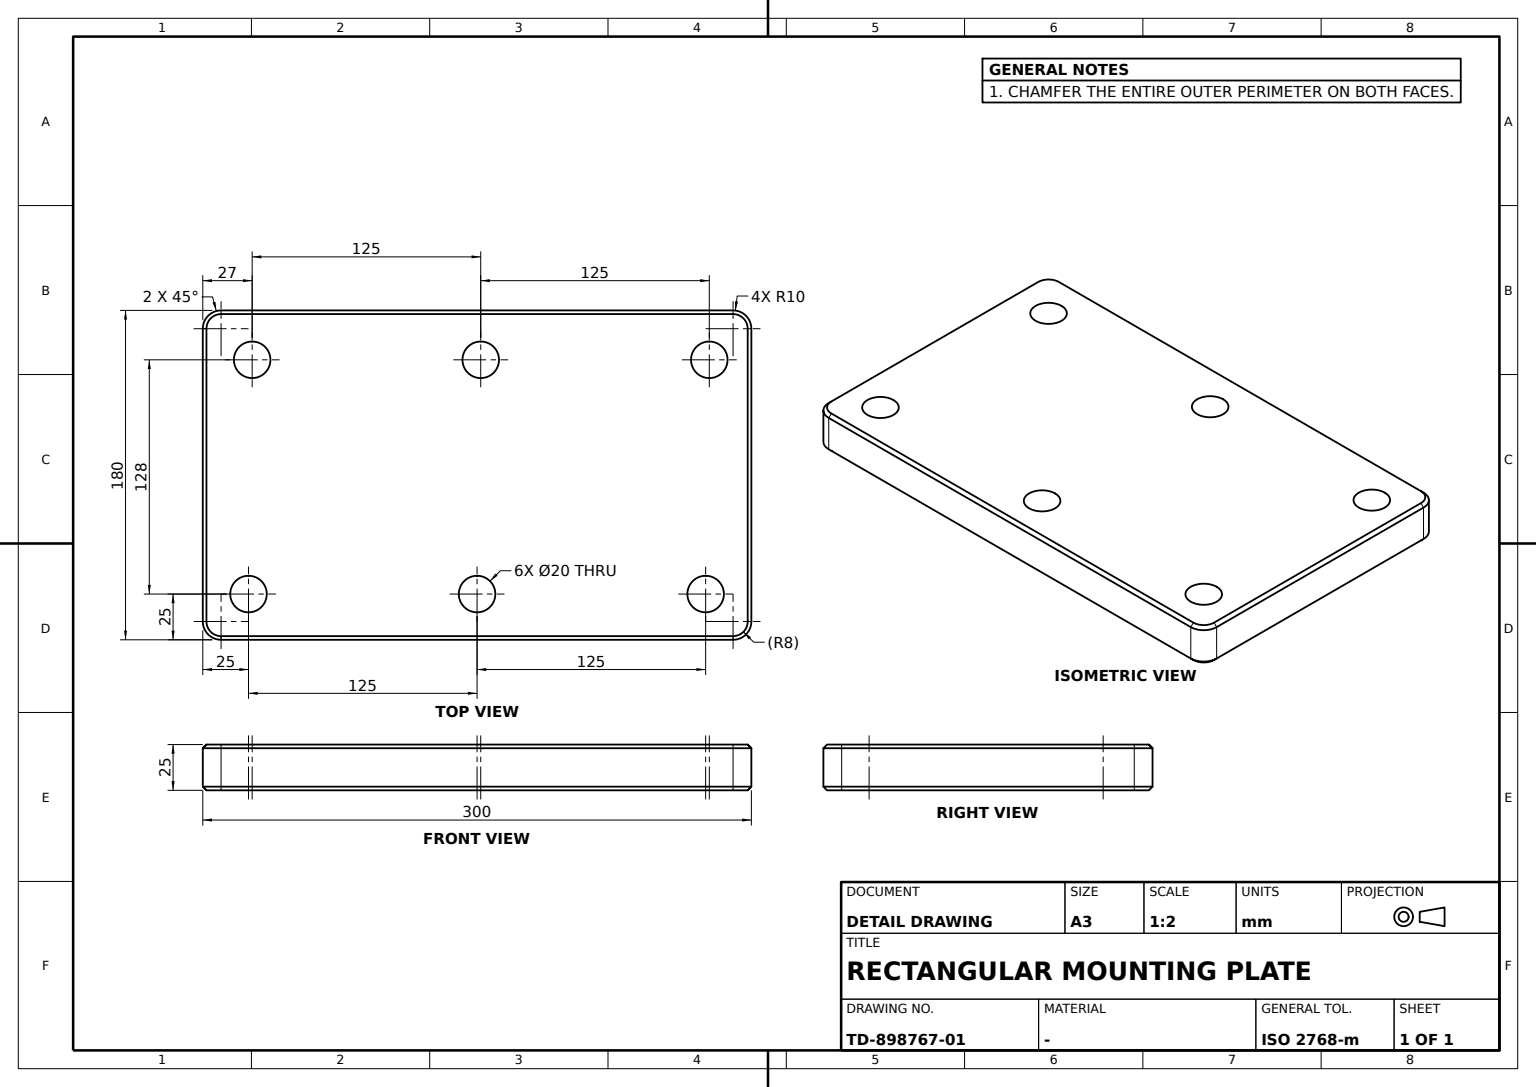
CATIA V5 part; units mm, degrees
sketch "Sketch1" plane through (0, 0, 0) normal (0, 0, -1) x (0, 1, 0)
  line L0 (-150, 90) -> (150, 90)
  line L1 (150, 90) -> (150, -90)
  line L2 (150, -90) -> (-150, -90)
  line L3 (-150, -90) -> (-150, 90)
  dimension "length L1" = 180
  dimension "length L0" = 300
  constraint horizontal L0 x-axis
  constraint horizontal L2 x-axis
  constraint vertical L1 y-axis
  constraint vertical L3 y-axis
  constraint symmetry L2 L0 x-axis
  constraint symmetry L1 L3 y-axis
extrude "Pad1" add sketch "Sketch1" along normal mid plane 25
fillet "Fillet1" radius 10 4 edges at (90, -150, 0) (90, 150, 0) (-90, -150, 0) (-90, 150, 0)
chamfer "Chamfer1" distance 2 angle 45 16 edges at (90, 0, 12.5) (87.0711, -147.0711, 12.5) (87.0711, 147.0711, 12.5) (0, -150, 12.5) (0, 150, 12.5) (-87.0711, -147.0711, 12.5) (-87.0711, 147.0711, 12.5) (-90, 0, 12.5) (90, 0, -12.5) (87.0711, -147.0711, -12.5) (87.0711, 147.0711, -12.5) (0, -150, -12.5) (0, 150, -12.5) (-87.0711, -147.0711, -12.5) (-87.0711, 147.0711, -12.5) (-90, 0, -12.5)
sketch "Sketch2" plane through (-66.3016, -121.8721, 12.5) normal (0, 0, 1) x (1, 0, 0)
  point P0 (3.3016, -1.1279)
  line L0 (-21.6984, -18.1279) -> (-21.6984, 261.8721) construction
  line L1 (146.3016, -26.1279) -> (-13.6984, -26.1279) construction
  dimension "distance P0 L0" = 25
  dimension "distance P0 L1" = 25
hole "Hole1" at (-63, -123, 12.5) direction (0, 0, -1) diameter 20 end through all
pattern_linear "RectPattern1" count 3 spacing 125 along (0, 1, 0) of "Hole1"
sketch "Sketch3" plane through (67.7941, -119.7449, 12.5) normal (0, 0, 1) x (1, 0, 0)
  point P0 (-2.7941, -5.2551)
  line L0 (12.2059, -30.2551) -> (-147.7941, -30.2551) construction
  line L1 (22.2059, 259.7449) -> (22.2059, -20.2551) construction
  dimension "distance P0 L0" = 25
  dimension "distance P0 L1" = 25
hole "Hole2" at (65, -125, 12.5) direction (0, 0, -1) diameter 20 end through all
pattern_linear "RectPattern2" count 3 spacing 125 along (0, 1, 0) of "Hole2"
